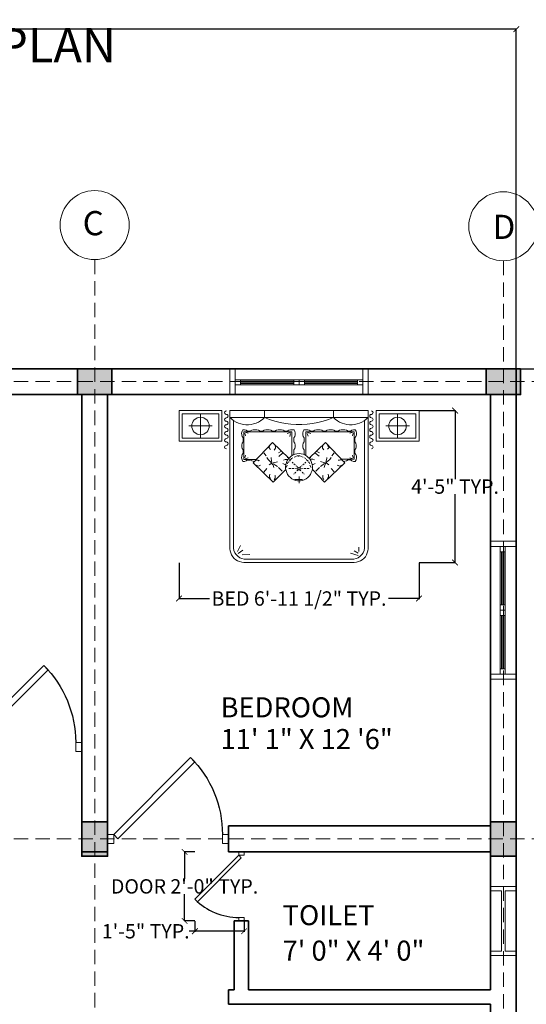
# Model space of a CAD drawing. Units: inches. Extents: x 782 to 2660, y -1008 to 166.
# Tile 10 of 12: x 1234 to 1410, y -176 to 166. Entities that reach past the tile are written whole.
import ezdxf

# ---------------------------------------------------------------- set-up
doc = ezdxf.new("R2010")
doc.units = ezdxf.units.IN
doc.header["$MEASUREMENT"] = 0
doc.linetypes.add('DASHED', pattern=[0.75, 0.5, -0.25])
for name, color, linetype, lineweight in [('A-ANNO-DIMS', 4, 'Continuous', 18), ('A-ANNO-TEXT', 4, 'Continuous', 18), ('A-AREA-IDEN', 4, 'Continuous', 18), ('A-COLS', 7, 'Continuous', 35), ('A-Door', 150, 'Continuous', 18), ('A-FURN', 8, 'Continuous', 13), ('A-Glaz', 4, 'Continuous', 18), ('A-GRID', 8, 'DASHED', 13), ('A-GRID-IDEN', 7, 'Continuous', 18), ('A-WALL', 7, 'Continuous', 35)]:
    doc.layers.add(name, color=color, linetype=linetype, lineweight=lineweight)
doc.layers.add('NET 01', color=8, linetype='Continuous')
doc.styles.get("Standard").update_dxf_attribs({"font": 'arial.ttf'})
doc.dimstyles.get("Standard").update_dxf_attribs({"dimtxt": 5, "dimasz": 2, "dimexe": 0.18, "dimexo": 0.0625, "dimgap": 0.09, "dimtad": 0, "dimtih": 1, "dimtoh": 1, "dimdec": 0, "dimzin": 0, "dimdsep": 46, "dimlunit": 3, "dimtxsty": 'Standard', "dimblk": 'ARCHTICK', "dimcen": 0.09, "dimadec": 0, "dimazin": 0, "dimtfac": 1, "dimtdec": 0, "dimtofl": 0, "dimtmove": 0, "dimatfit": 3, "dimfxl": 1, "dimtolj": 1, "dimtzin": 0, "dimarcsym": 0})

# ---------------------------------------------------------------- blocks, each defined once
blk = doc.blocks.new('A$C592222DF')
at = {"layer": 'A-Door'}
for points in [[(-0.0354, -0.0354), (-0.6718, 0.601), (-0.6364, 0.6364), (0, 0)], [(-0.95, 0), (-0.95, -0.075), (-0.9, -0.075), (-0.9, 0)], [(0, 0), (0, -0.075), (0.05, -0.075), (0.05, 0)]]:
    blk.add_lwpolyline(points, close=True, dxfattribs=at)
at = {"layer": 'NET 01'}
blk.add_arc((0, 0), 0.9, 135, 180, dxfattribs=at)
blk = doc.blocks.new('d-bed-4')
at = {"color": 0, "linetype": 'ByBlock'}
for p, q in [((0.56, 0), (0, 0)), ((0, 0), (0, -0.4)), ((0.56, -0.4), (0.56, 0)), ((0.664, -1.8), (0.664, 0)), ((0.664, 0), (2.464, 0)), ((0.664, 0), (2.464, 0)), ((0.664, -1.8), (0.664, 0)), ((1.114, 0), (1.114, -0.09)), ((2.014, 0), (2.014, -0.09)), ((2.464, 0), (2.464, -1.8)), ((2.464, 0), (2.464, -1.8)), ((2.568, -0.4), (2.568, 0)), ((2.568, 0), (3.128, 0)), ((3.128, 0), (3.128, -0.4)), ((0.52, -0.04), (0.04, -0.04)), ((0.04, -0.04), (0.04, -0.36)), ((0.28, -0.046), (0.28, -0.354)), ((0.52, -0.36), (0.52, -0.04)), ((2.464, -0.09), (0.664, -0.09)), ((0.664, -0.09), (0.689, -0.112)), ((0.689, -0.112), (0.716, -0.131)), ((0.709, -1.795), (0.709, -0.128)), ((1.064, -0.131), (1.091, -0.112)), ((1.091, -0.112), (1.114, -0.09)), ((1.114, -0.09), (1.181, -0.115)), ((1.181, -0.115), (1.249, -0.137)), ((1.879, -0.137), (1.947, -0.115)), ((1.947, -0.115), (2.014, -0.09)), ((2.014, -0.09), (2.037, -0.112)), ((2.037, -0.112), (2.064, -0.131)), ((2.412, -0.131), (2.439, -0.112)), ((2.419, -0.128), (2.419, -1.795)), ((2.439, -0.112), (2.464, -0.09)), ((2.608, -0.36), (2.608, -0.04)), ((2.608, -0.04), (3.088, -0.04)), ((2.848, -0.046), (2.848, -0.354)), ((3.088, -0.04), (3.088, -0.36)), ((0.126, -0.2), (0.434, -0.2)), ((0.716, -0.131), (0.745, -0.148)), ((0.745, -0.148), (0.776, -0.162)), ((0.776, -0.162), (0.806, -0.173)), ((0.806, -0.173), (0.84, -0.18)), ((0.821, -0.268), (0.831, -0.248)), ((0.831, -0.248), (0.853, -0.248)), ((0.84, -0.18), (0.873, -0.184)), ((0.853, -0.248), (0.875, -0.256)), ((0.873, -0.184), (0.907, -0.184)), ((0.875, -0.256), (0.894, -0.266)), ((0.907, -0.184), (0.939, -0.18)), ((0.925, -0.266), (0.947, -0.256)), ((0.939, -0.18), (0.972, -0.173)), ((0.947, -0.256), (0.968, -0.25)), ((0.968, -0.25), (0.99, -0.248)), ((0.972, -0.173), (1.004, -0.162)), ((0.99, -0.248), (1.013, -0.25)), ((1.004, -0.162), (1.035, -0.148)), ((1.013, -0.25), (1.035, -0.256)), ((1.035, -0.148), (1.064, -0.131)), ((1.035, -0.256), (1.056, -0.266)), ((1.087, -0.266), (1.109, -0.256)), ((1.109, -0.256), (1.13, -0.25)), ((1.13, -0.25), (1.152, -0.248)), ((1.152, -0.248), (1.175, -0.25)), ((1.175, -0.25), (1.197, -0.256)), ((1.197, -0.256), (1.217, -0.266)), ((1.249, -0.137), (1.317, -0.155)), ((1.249, -0.266), (1.269, -0.256)), ((1.269, -0.256), (1.29, -0.25)), ((1.29, -0.25), (1.314, -0.248)), ((1.314, -0.248), (1.337, -0.25)), ((1.317, -0.155), (1.388, -0.169)), ((1.337, -0.25), (1.359, -0.256)), ((1.359, -0.256), (1.379, -0.266)), ((1.388, -0.169), (1.458, -0.178)), ((1.411, -0.266), (1.431, -0.256)), ((1.431, -0.256), (1.451, -0.248)), ((1.451, -0.248), (1.474, -0.248)), ((1.458, -0.178), (1.528, -0.182)), ((1.474, -0.248), (1.501, -0.248)), ((1.501, -0.248), (1.51, -0.268)), ((1.528, -0.182), (1.6, -0.182)), ((1.6, -0.182), (1.67, -0.178)), ((1.627, -0.248), (1.618, -0.268)), ((1.654, -0.248), (1.627, -0.248)), ((1.677, -0.248), (1.654, -0.248)), ((1.67, -0.178), (1.74, -0.169)), ((1.697, -0.256), (1.677, -0.248)), ((1.717, -0.266), (1.697, -0.256)), ((1.74, -0.169), (1.811, -0.155)), ((1.769, -0.256), (1.749, -0.266)), ((1.791, -0.25), (1.769, -0.256)), ((1.814, -0.248), (1.791, -0.25)), ((1.811, -0.155), (1.879, -0.137)), ((1.838, -0.25), (1.814, -0.248)), ((1.859, -0.256), (1.838, -0.25)), ((1.879, -0.266), (1.859, -0.256)), ((1.931, -0.256), (1.911, -0.266)), ((1.953, -0.25), (1.931, -0.256)), ((1.976, -0.248), (1.953, -0.25)), ((1.998, -0.25), (1.976, -0.248)), ((2.019, -0.256), (1.998, -0.25)), ((2.041, -0.266), (2.019, -0.256)), ((2.064, -0.131), (2.093, -0.148)), ((2.093, -0.256), (2.072, -0.266)), ((2.093, -0.148), (2.124, -0.162)), ((2.115, -0.25), (2.093, -0.256)), ((2.138, -0.248), (2.115, -0.25)), ((2.124, -0.162), (2.156, -0.173)), ((2.16, -0.25), (2.138, -0.248)), ((2.156, -0.173), (2.189, -0.18)), ((2.181, -0.256), (2.16, -0.25)), ((2.203, -0.266), (2.181, -0.256)), ((2.189, -0.18), (2.221, -0.184)), ((2.221, -0.184), (2.255, -0.184)), ((2.253, -0.256), (2.234, -0.266)), ((2.275, -0.248), (2.253, -0.256)), ((2.255, -0.184), (2.288, -0.18)), ((2.297, -0.248), (2.275, -0.248)), ((2.288, -0.18), (2.322, -0.173)), ((2.307, -0.268), (2.297, -0.248)), ((2.322, -0.173), (2.352, -0.162)), ((2.352, -0.162), (2.383, -0.148)), ((2.383, -0.148), (2.412, -0.131)), ((3.002, -0.2), (2.694, -0.2)), ((0.04, -0.36), (0.52, -0.36)), ((0.815, -0.292), (0.821, -0.268)), ((0.817, -0.315), (0.815, -0.292)), ((0.824, -0.337), (0.817, -0.315)), ((0.835, -0.356), (0.824, -0.337)), ((0.835, -0.405), (0.835, -0.356)), ((0.844, -0.635), (0.844, -0.275)), ((0.844, -0.275), (1.472, -0.275)), ((0.857, -0.293), (0.866, -0.329)), ((0.862, -0.281), (0.902, -0.293)), ((0.894, -0.266), (0.925, -0.266)), ((1.056, -0.266), (1.087, -0.266)), ((1.217, -0.266), (1.249, -0.266)), ((1.379, -0.266), (1.411, -0.266)), ((1.451, -0.284), (1.409, -0.299)), ((1.454, -0.299), (1.445, -0.335)), ((1.472, -0.275), (1.472, -0.581)), ((1.508, -0.337), (1.496, -0.356)), ((1.496, -0.356), (1.496, -0.405)), ((1.515, -0.315), (1.508, -0.337)), ((1.51, -0.268), (1.515, -0.292)), ((1.515, -0.292), (1.515, -0.315)), ((1.618, -0.268), (1.613, -0.292)), ((1.613, -0.292), (1.613, -0.315)), ((1.613, -0.315), (1.62, -0.337)), ((1.62, -0.337), (1.632, -0.356)), ((1.632, -0.356), (1.632, -0.405)), ((2.282, -0.274), (1.654, -0.274)), ((1.654, -0.274), (1.654, -0.58)), ((1.672, -0.297), (1.681, -0.333)), ((1.676, -0.283), (1.717, -0.297)), ((1.749, -0.266), (1.717, -0.266)), ((1.911, -0.266), (1.879, -0.266)), ((2.072, -0.266), (2.041, -0.266)), ((2.234, -0.266), (2.203, -0.266)), ((2.264, -0.279), (2.225, -0.292)), ((2.27, -0.292), (2.261, -0.328)), ((2.282, -0.634), (2.282, -0.274)), ((2.293, -0.356), (2.304, -0.337)), ((2.293, -0.405), (2.293, -0.356)), ((2.304, -0.337), (2.311, -0.315)), ((2.313, -0.292), (2.307, -0.268)), ((2.311, -0.315), (2.313, -0.292)), ((3.088, -0.36), (2.608, -0.36)), ((0, -0.4), (0.56, -0.4)), ((0.819, -0.448), (0.824, -0.425)), ((0.819, -0.47), (0.819, -0.448)), ((0.824, -0.493), (0.819, -0.47)), ((0.824, -0.425), (0.835, -0.405)), ((0.835, -0.513), (0.824, -0.493)), ((0.835, -0.553), (0.835, -0.513)), ((0.965, -0.68), (1.217, -0.416)), ((1.19, -0.452), (1.172, -0.482)), ((1.172, -0.482), (1.193, -0.506)), ((1.217, -0.416), (1.433, -0.621)), ((1.256, -0.491), (1.238, -0.515)), ((1.253, -0.446), (1.256, -0.491)), ((1.496, -0.405), (1.508, -0.425)), ((1.508, -0.493), (1.496, -0.513)), ((1.496, -0.513), (1.496, -0.567)), ((1.508, -0.425), (1.514, -0.448)), ((1.514, -0.47), (1.508, -0.493)), ((1.514, -0.448), (1.514, -0.47)), ((1.62, -0.425), (1.614, -0.448)), ((1.614, -0.448), (1.614, -0.47)), ((1.614, -0.47), (1.62, -0.493)), ((1.632, -0.405), (1.62, -0.425)), ((1.62, -0.493), (1.632, -0.513)), ((1.632, -0.513), (1.632, -0.567)), ((1.91, -0.414), (1.694, -0.619)), ((1.874, -0.445), (1.87, -0.49)), ((1.87, -0.49), (1.888, -0.513)), ((2.162, -0.679), (1.91, -0.414)), ((1.955, -0.481), (1.933, -0.504)), ((1.937, -0.45), (1.955, -0.481)), ((2.304, -0.425), (2.293, -0.405)), ((2.293, -0.513), (2.304, -0.493)), ((2.293, -0.553), (2.293, -0.513)), ((2.309, -0.448), (2.304, -0.425)), ((2.304, -0.493), (2.309, -0.47)), ((2.309, -0.47), (2.309, -0.448)), ((3.128, -0.4), (2.568, -0.4)), ((0.815, -0.617), (0.817, -0.594)), ((0.821, -0.641), (0.815, -0.617)), ((0.817, -0.594), (0.824, -0.572)), ((0.831, -0.661), (0.821, -0.641)), ((0.824, -0.572), (0.835, -0.553)), ((1.01, -0.635), (0.844, -0.635)), ((0.857, -0.617), (0.866, -0.581)), ((0.862, -0.63), (0.902, -0.617)), ((1.105, -0.551), (1.136, -0.59)), ((1.163, -0.639), (1.145, -0.612)), ((1.202, -0.675), (1.163, -0.639)), ((1.199, -0.626), (1.199, -0.612)), ((1.211, -0.675), (1.199, -0.626)), ((1.328, -0.533), (1.298, -0.551)), ((1.355, -0.551), (1.301, -0.596)), ((1.382, -0.635), (1.361, -0.644)), ((1.415, -0.635), (1.382, -0.635)), ((1.409, -0.612), (1.433, -0.621)), ((1.411, -0.652), (1.425, -0.63)), ((1.415, -0.635), (1.418, -0.639)), ((1.425, -0.63), (1.443, -0.61)), ((1.465, -0.626), (1.438, -0.659)), ((1.438, -0.635), (1.442, -0.641)), ((1.443, -0.61), (1.463, -0.592)), ((1.463, -0.592), (1.487, -0.578)), ((1.465, -0.626), (1.483, -0.617)), ((1.487, -0.578), (1.512, -0.567)), ((1.528, -0.596), (1.501, -0.608)), ((1.512, -0.567), (1.537, -0.562)), ((1.537, -0.562), (1.564, -0.558)), ((1.537, -0.59), (1.562, -0.59)), ((1.58, -0.59), (1.555, -0.59)), ((1.559, -0.587), (1.559, -0.599)), ((1.559, -0.587), (1.559, -0.599)), ((1.564, -0.558), (1.591, -0.562)), ((1.589, -0.596), (1.616, -0.608)), ((1.591, -0.562), (1.616, -0.567)), ((1.616, -0.567), (1.641, -0.578)), ((1.652, -0.626), (1.634, -0.617)), ((1.641, -0.578), (1.665, -0.592)), ((1.659, -0.635), (1.681, -0.657)), ((1.665, -0.592), (1.685, -0.61)), ((1.685, -0.61), (1.703, -0.63)), ((1.717, -0.61), (1.694, -0.619)), ((1.703, -0.63), (1.717, -0.652)), ((1.712, -0.634), (1.708, -0.637)), ((1.712, -0.634), (1.744, -0.634)), ((1.744, -0.634), (1.766, -0.643)), ((1.771, -0.549), (1.825, -0.594)), ((1.798, -0.531), (1.829, -0.549)), ((1.915, -0.673), (1.928, -0.625)), ((1.924, -0.673), (1.964, -0.637)), ((1.928, -0.625), (1.928, -0.61)), ((1.964, -0.637), (1.982, -0.61)), ((2.021, -0.549), (1.991, -0.589)), ((2.117, -0.634), (2.282, -0.634)), ((2.264, -0.628), (2.225, -0.616)), ((2.27, -0.616), (2.261, -0.58)), ((2.304, -0.572), (2.293, -0.553)), ((2.297, -0.661), (2.307, -0.641)), ((2.311, -0.594), (2.304, -0.572)), ((2.307, -0.641), (2.313, -0.617)), ((2.313, -0.617), (2.311, -0.594)), ((0.853, -0.661), (0.831, -0.661)), ((0.875, -0.653), (0.853, -0.661)), ((0.894, -0.643), (0.875, -0.653)), ((0.907, -0.644), (0.893, -0.644)), ((0.925, -0.643), (0.894, -0.643)), ((0.916, -0.644), (0.907, -0.644)), ((0.925, -0.644), (0.916, -0.644)), ((0.947, -0.653), (0.925, -0.643)), ((0.968, -0.659), (0.947, -0.653)), ((1.229, -0.932), (0.965, -0.68)), ((0.983, -0.661), (0.968, -0.659)), ((1.006, -0.644), (1.024, -0.644)), ((1.006, -0.711), (1.037, -0.725)), ((1.024, -0.644), (1.042, -0.653)), ((1.042, -0.653), (1.028, -0.644)), ((1.028, -0.644), (1.051, -0.648)), ((1.037, -0.725), (1.055, -0.716)), ((1.055, -0.716), (1.064, -0.711)), ((1.105, -0.801), (1.145, -0.756)), ((1.175, -0.707), (1.208, -0.684)), ((1.22, -0.707), (1.211, -0.675)), ((1.226, -0.68), (1.283, -0.666)), ((1.226, -0.711), (1.235, -0.743)), ((1.229, -0.693), (1.283, -0.729)), ((1.343, -0.788), (1.298, -0.743)), ((1.379, -0.702), (1.352, -0.689)), ((1.379, -0.702), (1.391, -0.702)), ((1.389, -0.729), (1.393, -0.702)), ((1.389, -0.756), (1.389, -0.729)), ((1.395, -0.781), (1.389, -0.756)), ((1.393, -0.702), (1.4, -0.677)), ((1.397, -0.743), (1.411, -0.711)), ((1.4, -0.677), (1.411, -0.652)), ((1.42, -0.677), (1.415, -0.695)), ((1.42, -0.677), (1.429, -0.668)), ((1.46, -0.756), (1.429, -0.756)), ((1.487, -0.686), (1.474, -0.671)), ((1.496, -0.756), (1.474, -0.756)), ((1.514, -0.707), (1.496, -0.695)), ((1.514, -0.756), (1.51, -0.756)), ((1.532, -0.72), (1.523, -0.72)), ((1.55, -0.765), (1.523, -0.756)), ((1.559, -0.747), (1.537, -0.729)), ((1.55, -0.756), (1.55, -0.747)), ((1.55, -0.747), (1.559, -0.747)), ((1.55, -0.765), (1.55, -0.756)), ((1.559, -0.77), (1.55, -0.765)), ((1.559, -0.747), (1.562, -0.745)), ((1.568, -0.747), (1.562, -0.745)), ((1.568, -0.747), (1.589, -0.729)), ((1.577, -0.747), (1.568, -0.747)), ((1.568, -0.77), (1.577, -0.765)), ((1.577, -0.756), (1.577, -0.747)), ((1.577, -0.765), (1.577, -0.756)), ((1.577, -0.765), (1.604, -0.756)), ((1.595, -0.72), (1.604, -0.72)), ((1.613, -0.707), (1.631, -0.695)), ((1.613, -0.756), (1.616, -0.756)), ((1.631, -0.756), (1.652, -0.756)), ((1.64, -0.686), (1.652, -0.671)), ((1.667, -0.756), (1.697, -0.756)), ((1.697, -0.677), (1.688, -0.668)), ((1.697, -0.677), (1.703, -0.695)), ((1.721, -0.743), (1.706, -0.711)), ((1.717, -0.652), (1.728, -0.677)), ((1.728, -0.677), (1.735, -0.702)), ((1.739, -0.756), (1.733, -0.781)), ((1.748, -0.7), (1.735, -0.7)), ((1.735, -0.702), (1.739, -0.729)), ((1.739, -0.729), (1.739, -0.756)), ((1.897, -0.931), (1.739, -0.769)), ((1.748, -0.7), (1.775, -0.688)), ((1.784, -0.787), (1.829, -0.742)), ((1.901, -0.679), (1.843, -0.664)), ((1.897, -0.691), (1.843, -0.727)), ((1.901, -0.709), (1.892, -0.742)), ((1.897, -0.931), (2.162, -0.679)), ((1.906, -0.706), (1.915, -0.673)), ((1.951, -0.706), (1.919, -0.682)), ((2.021, -0.799), (1.982, -0.754)), ((2.072, -0.715), (2.063, -0.709)), ((2.09, -0.724), (2.072, -0.715)), ((2.099, -0.643), (2.075, -0.646)), ((2.102, -0.643), (2.084, -0.652)), ((2.084, -0.652), (2.099, -0.643)), ((2.12, -0.709), (2.09, -0.724)), ((2.12, -0.643), (2.102, -0.643)), ((2.145, -0.661), (2.16, -0.659)), ((2.16, -0.659), (2.181, -0.653)), ((2.181, -0.653), (2.203, -0.643)), ((2.201, -0.643), (2.21, -0.643)), ((2.203, -0.643), (2.234, -0.643)), ((2.21, -0.643), (2.219, -0.643)), ((2.219, -0.643), (2.234, -0.643)), ((2.234, -0.643), (2.253, -0.653)), ((2.253, -0.653), (2.275, -0.661)), ((2.275, -0.661), (2.297, -0.661)), ((1.181, -0.851), (1.184, -0.828)), ((1.181, -0.869), (1.181, -0.851)), ((1.193, -0.891), (1.181, -0.869)), ((1.229, -0.932), (1.388, -0.77)), ((1.238, -0.9), (1.253, -0.882)), ((1.253, -0.846), (1.247, -0.846)), ((1.253, -0.882), (1.253, -0.846)), ((1.404, -0.808), (1.395, -0.781)), ((1.415, -0.832), (1.404, -0.808)), ((1.431, -0.853), (1.415, -0.832)), ((1.451, -0.873), (1.431, -0.853)), ((1.47, -0.889), (1.451, -0.873)), ((1.496, -0.902), (1.47, -0.889)), ((1.501, -0.819), (1.496, -0.828)), ((1.609, -0.896), (1.503, -0.896)), ((1.523, -0.801), (1.51, -0.815)), ((1.532, -0.792), (1.532, -0.792)), ((1.559, -0.77), (1.537, -0.783)), ((1.559, -0.77), (1.562, -0.77)), ((1.568, -0.77), (1.562, -0.77)), ((1.564, -0.945), (1.564, -0.86)), ((1.568, -0.77), (1.589, -0.783)), ((1.595, -0.792), (1.595, -0.792)), ((1.604, -0.801), (1.616, -0.815)), ((1.625, -0.819), (1.631, -0.828)), ((1.658, -0.889), (1.632, -0.902)), ((1.677, -0.873), (1.658, -0.889)), ((1.697, -0.853), (1.677, -0.873)), ((1.713, -0.832), (1.697, -0.853)), ((1.724, -0.808), (1.713, -0.832)), ((1.733, -0.781), (1.724, -0.808)), ((1.874, -0.88), (1.874, -0.844)), ((1.874, -0.844), (1.879, -0.844)), ((1.888, -0.898), (1.874, -0.88)), ((1.933, -0.889), (1.946, -0.868)), ((1.946, -0.85), (1.942, -0.826)), ((1.946, -0.868), (1.946, -0.85)), ((1.521, -0.911), (1.496, -0.902)), ((1.546, -0.916), (1.521, -0.911)), ((1.564, -0.916), (1.546, -0.916)), ((1.582, -0.916), (1.564, -0.916)), ((1.607, -0.911), (1.582, -0.916)), ((1.632, -0.902), (1.607, -0.911)), ((0.716, -1.825), (0.709, -1.795)), ((0.763, -1.836), (0.803, -1.76)), ((2.342, -1.836), (2.342, -1.778)), ((2.419, -1.795), (2.412, -1.825)), ((0.668, -1.827), (0.664, -1.8)), ((0.668, -1.827), (0.664, -1.8)), ((0.675, -1.854), (0.668, -1.827)), ((0.675, -1.854), (0.668, -1.827)), ((0.686, -1.881), (0.675, -1.854)), ((0.686, -1.881), (0.675, -1.854)), ((0.7, -1.904), (0.686, -1.881)), ((0.7, -1.904), (0.686, -1.881)), ((0.718, -1.926), (0.7, -1.904)), ((0.718, -1.926), (0.7, -1.904)), ((0.727, -1.852), (0.716, -1.825)), ((0.745, -1.877), (0.727, -1.852)), ((0.767, -1.899), (0.745, -1.877)), ((0.792, -1.917), (0.767, -1.899)), ((0.772, -1.863), (0.83, -1.818)), ((0.819, -1.928), (0.792, -1.917)), ((0.821, -1.881), (0.925, -1.876)), ((2.333, -1.89), (2.234, -1.858)), ((2.333, -1.858), (2.282, -1.827)), ((2.336, -1.917), (2.309, -1.928)), ((2.361, -1.899), (2.336, -1.917)), ((2.383, -1.877), (2.361, -1.899)), ((2.401, -1.852), (2.383, -1.877)), ((2.412, -1.825), (2.401, -1.852)), ((2.428, -1.904), (2.41, -1.926)), ((2.428, -1.904), (2.41, -1.926)), ((2.442, -1.881), (2.428, -1.904)), ((2.442, -1.881), (2.428, -1.904)), ((2.453, -1.854), (2.442, -1.881)), ((2.453, -1.854), (2.442, -1.881)), ((2.46, -1.827), (2.453, -1.854)), ((2.46, -1.827), (2.453, -1.854)), ((2.464, -1.8), (2.46, -1.827)), ((2.464, -1.8), (2.46, -1.827)), ((0.74, -1.944), (0.718, -1.926)), ((0.74, -1.944), (0.718, -1.926)), ((0.763, -1.958), (0.74, -1.944)), ((0.763, -1.958), (0.74, -1.944)), ((0.79, -1.969), (0.763, -1.958)), ((0.79, -1.969), (0.763, -1.958)), ((0.817, -1.976), (0.79, -1.969)), ((0.817, -1.976), (0.79, -1.969)), ((0.844, -1.98), (0.817, -1.976)), ((0.844, -1.98), (0.817, -1.976)), ((0.849, -1.935), (0.819, -1.928)), ((2.284, -1.98), (0.844, -1.98)), ((2.284, -1.98), (0.844, -1.98)), ((2.279, -1.935), (0.849, -1.935)), ((2.309, -1.928), (2.279, -1.935)), ((2.311, -1.976), (2.284, -1.98)), ((2.311, -1.976), (2.284, -1.98)), ((2.338, -1.969), (2.311, -1.976)), ((2.338, -1.969), (2.311, -1.976)), ((2.365, -1.958), (2.338, -1.969)), ((2.365, -1.958), (2.338, -1.969)), ((2.388, -1.944), (2.365, -1.958)), ((2.388, -1.944), (2.365, -1.958)), ((2.41, -1.926), (2.388, -1.944)), ((2.41, -1.926), (2.388, -1.944))]:
    blk.add_line(p, q, dxfattribs=at)
for centre in [(0.28, -0.2), (2.848, -0.2)]:
    blk.add_ellipse(centre, major_axis=(-0.0806, 0.0806), ratio=1, dxfattribs=at)
for centre, major_axis, start_param, end_param in [((0.617, -0.026), (-0.0159, 0.0159), 5.497787, 8.63938), ((0.617, -0.116), (-0.0159, 0.0159), 5.497787, 8.63938), ((0.617, -0.071), (-0.0159, 0.0159), 2.356194, 5.497787), ((2.507, -0.071), (0.0159, 0.0159), 0.785398, 3.926991), ((2.507, -0.026), (0.0159, 0.0159), 3.926991, 7.068583), ((2.507, -0.116), (0.0159, 0.0159), 3.926991, 7.068583), ((0.617, -0.206), (-0.0159, 0.0159), 5.497787, 8.63938), ((0.617, -0.161), (-0.0159, 0.0159), 2.356194, 5.497787), ((0.617, -0.161), (-0.0159, 0.0159), 2.356194, 5.497787), ((0.617, -0.251), (-0.0159, 0.0159), 2.356194, 5.497787), ((2.507, -0.161), (0.0159, 0.0159), 0.785398, 3.926991), ((2.507, -0.161), (0.0159, 0.0159), 0.785398, 3.926991), ((2.507, -0.251), (0.0159, 0.0159), 0.785398, 3.926991), ((2.507, -0.206), (0.0159, 0.0159), 3.926991, 7.068583), ((0.617, -0.296), (-0.0159, 0.0159), 5.497787, 8.63938), ((0.617, -0.386), (-0.0159, 0.0159), 5.497787, 8.63938), ((0.617, -0.341), (-0.0159, 0.0159), 2.356194, 5.497787), ((2.507, -0.341), (0.0159, 0.0159), 0.785398, 3.926991), ((2.507, -0.296), (0.0159, 0.0159), 3.926991, 7.068583), ((2.507, -0.386), (0.0159, 0.0159), 3.926991, 7.068583), ((0.617, -0.476), (-0.0159, 0.0159), 5.497787, 8.63938), ((0.617, -0.431), (-0.0159, 0.0159), 2.356194, 5.497787), ((2.507, -0.431), (0.0159, 0.0159), 0.785398, 3.926991), ((2.507, -0.476), (0.0159, 0.0159), 3.926991, 7.068583)]:
    blk.add_ellipse(centre, major_axis=major_axis, ratio=1, start_param=start_param, end_param=end_param, dxfattribs=at)
blk = doc.blocks.new('WIN-48-FRAME-A')
for p, q in [((0, 48), (0, 0)), ((0, 48), (9, 48)), ((9, 48), (0, 48)), ((9, 48), (9, 0)), ((9, 46.15), (0, 46.15)), ((9, 46.15), (0, 46.15)), ((9, 46.15), (0, 46.15)), ((3.35, 1.85), (3.35, 46.15)), ((5.19, 1.85), (5.19, 46.15)), ((5.19, 44.31), (3.35, 44.31)), ((3.9, 44.31), (3.9, 25.85)), ((4.27, 44.31), (4.27, 25.85)), ((4.64, 44.31), (4.64, 25.85)), ((3.35, 25.85), (5.19, 25.85)), ((3.35, 24), (5.19, 24)), ((3.35, 22.15), (5.19, 22.15)), ((3.9, 3.69), (3.9, 22.15)), ((4.27, 3.69), (4.27, 22.15)), ((4.64, 3.69), (4.64, 22.15)), ((5.19, 3.69), (3.35, 3.69)), ((9, 1.85), (0, 1.85)), ((9, 1.85), (0, 1.85)), ((0, 0), (9, 0)), ((0, 0), (9, 0))]:
    blk.add_line(p, q)
blk = doc.blocks.new('WIN-24')
for p, q in [((0, 0), (0, 24)), ((0, 24), (9, 24)), ((9, 24), (9, 0)), ((0, 22.49), (3.9, 22.49)), ((3.9, 1.51), (3.9, 22.49)), ((5.1, 22.49), (9, 22.49)), ((5.1, 1.51), (5.1, 22.49)), ((3.9, 1.51), (0, 1.51)), ((9, 0), (0, 0)), ((9, 1.51), (5.1, 1.51))]:
    blk.add_line(p, q)
blk = doc.blocks.new('COL-9X12')
h = blk.add_hatch(color=256)
h.dxf.hatch_style = 1
h.paths.add_polyline_path([(9, 12), (0, 12), (0, 0), (9, 0)])
blk.add_lwpolyline([(0, 12), (9, 12), (9, 0), (0, 0)], close=True)
blk = doc.blocks.new('_ArchTick')
at = {"color": 0, "linetype": 'ByBlock', "const_width": 0.15}
blk.add_lwpolyline([(-0.5, -0.5), (0.5, 0.5)], dxfattribs=at)
blk = doc.blocks.new('*D29')
at = {"layer": 'A-ANNO-DIMS', "color": 0, "lineweight": -2, "transparency": 16777216}
for p, q in [((1294.95, -122.99), (1291.23, -122.99)), ((1291.41, -122.99), (1291.41, -132.32)), ((1291.41, -146.99), (1291.41, -137.67)), ((1294.95, -146.99), (1291.23, -146.99))]:
    blk.add_line(p, q, dxfattribs=at)
at = {"layer": 'Defpoints', "color": 0, "transparency": 16777216}
for p in [(1291.41, -122.99), (1295.01, -122.99), (1295.01, -146.99)]:
    blk.add_point(p, dxfattribs=at)
at = {"layer": 'A-ANNO-DIMS', "color": 0, "lineweight": -2, "transparency": 16777216, "xscale": 2, "yscale": 2, "zscale": 2}
for p, rotation in [((1291.41, -122.99), 90), ((1291.41, -146.99), 270)]:
    blk.add_blockref('_ArchTick', p, dxfattribs=dict(at, rotation=rotation))
at = {"layer": 'A-ANNO-DIMS', "color": 0, "transparency": 16777216, "insert": (1291.41, -134.99), "char_height": 5, "attachment_point": 5}
blk.add_mtext('\\A1;DOOR 2\'-0" TYP.', dxfattribs=at)
blk = doc.blocks.new('*D30')
at = {"layer": 'A-ANNO-DIMS', "color": 0, "lineweight": -2, "transparency": 16777216}
for p, q in [((1295.01, -147.06), (1295.01, -150.77)), ((1312.08, -147.06), (1312.08, -150.77)), ((1295.01, -150.59), (1293.01, -150.59)), ((1312.08, -150.59), (1295.01, -150.59))]:
    blk.add_line(p, q, dxfattribs=at)
at = {"layer": 'Defpoints', "color": 0, "transparency": 16777216}
for p in [(1295.01, -146.99), (1312.08, -146.99), (1295.01, -150.59)]:
    blk.add_point(p, dxfattribs=at)
at = {"layer": 'A-ANNO-DIMS', "color": 0, "lineweight": -2, "transparency": 16777216, "xscale": 2, "yscale": 2, "zscale": 2, "rotation": 180}
blk.add_blockref('_ArchTick', (1295.01, -150.59), dxfattribs=at)
at = {"layer": 'A-ANNO-DIMS', "color": 0, "lineweight": -2, "transparency": 16777216, "xscale": 2, "yscale": 2, "zscale": 2}
blk.add_blockref('_ArchTick', (1312.08, -150.59), dxfattribs=at)
at = {"layer": 'A-ANNO-DIMS', "color": 0, "transparency": 16777216, "insert": (1277.92, -150.59), "char_height": 5, "attachment_point": 5}
blk.add_mtext('\\A1;1\'-5" TYP.', dxfattribs=at)
blk = doc.blocks.new('*D41')
at = {"layer": 'A-ANNO-DIMS', "color": 0, "lineweight": -2, "transparency": 16777216}
for p, q in [((1289.48, -22.44), (1289.48, -35.07)), ((1372.89, -22.44), (1372.89, -35.07)), ((1289.48, -34.89), (1300.05, -34.89)), ((1372.89, -34.89), (1362.32, -34.89))]:
    blk.add_line(p, q, dxfattribs=at)
at = {"layer": 'Defpoints', "color": 0, "transparency": 16777216}
for p in [(1289.48, -22.37), (1372.89, -22.37), (1372.89, -34.89)]:
    blk.add_point(p, dxfattribs=at)
at = {"layer": 'A-ANNO-DIMS', "color": 0, "lineweight": -2, "transparency": 16777216, "xscale": 2, "yscale": 2, "zscale": 2, "rotation": 180}
blk.add_blockref('_ArchTick', (1289.48, -34.89), dxfattribs=at)
at = {"layer": 'A-ANNO-DIMS', "color": 0, "lineweight": -2, "transparency": 16777216, "xscale": 2, "yscale": 2, "zscale": 2}
blk.add_blockref('_ArchTick', (1372.89, -34.89), dxfattribs=at)
at = {"layer": 'A-ANNO-DIMS', "color": 0, "transparency": 16777216, "insert": (1331.18, -34.89), "char_height": 5, "attachment_point": 5}
blk.add_mtext('\\A1;BED 6\'-11 1/2" TYP.', dxfattribs=at)
blk = doc.blocks.new('*D42')
at = {"layer": 'A-ANNO-DIMS', "color": 0, "lineweight": -2, "transparency": 16777216}
for p, q in [((1372.95, 30.43), (1385.58, 30.43)), ((1385.4, 30.43), (1385.4, 6.66)), ((1385.4, -22.37), (1385.4, 1.39)), ((1372.95, -22.37), (1385.58, -22.37))]:
    blk.add_line(p, q, dxfattribs=at)
at = {"layer": 'Defpoints', "color": 0, "transparency": 16777216}
for p in [(1372.89, 30.43), (1385.4, 30.43), (1372.89, -22.37)]:
    blk.add_point(p, dxfattribs=at)
at = {"layer": 'A-ANNO-DIMS', "color": 0, "lineweight": -2, "transparency": 16777216, "xscale": 2, "yscale": 2, "zscale": 2}
for p, rotation in [((1385.4, 30.43), 90), ((1385.4, -22.37), 270)]:
    blk.add_blockref('_ArchTick', p, dxfattribs=dict(at, rotation=rotation))
at = {"layer": 'A-ANNO-DIMS', "color": 0, "transparency": 16777216, "insert": (1385.4, 4.03), "char_height": 5, "attachment_point": 5}
blk.add_mtext('\\A1;4\'-5" TYP.', dxfattribs=at)
blk = doc.blocks.new('*D51')
at = {"layer": 'A-ANNO-DIMS', "color": 0, "lineweight": -2, "transparency": 16777216}
for p, q in [((1406.75, 45.01), (1579.89, 45.01)), ((1579.71, 45.01), (1579.71, -327.35)), ((1579.71, -704.99), (1579.71, -332.64)), ((1406.75, -704.99), (1579.89, -704.99))]:
    blk.add_line(p, q, dxfattribs=at)
at = {"layer": 'Defpoints', "color": 0, "transparency": 16777216}
for p in [(1406.68, 45.01), (1579.71, 45.01), (1406.68, -704.99)]:
    blk.add_point(p, dxfattribs=at)
at = {"layer": 'A-ANNO-DIMS', "color": 0, "lineweight": -2, "transparency": 16777216, "xscale": 2, "yscale": 2, "zscale": 2}
for p, rotation in [((1579.71, 45.01), 90), ((1579.71, -704.99), 270)]:
    blk.add_blockref('_ArchTick', p, dxfattribs=dict(at, rotation=rotation))
at = {"layer": 'A-ANNO-DIMS', "color": 0, "transparency": 16777216, "insert": (1579.71, -329.99), "char_height": 5, "attachment_point": 5}
blk.add_mtext('\\A1;62\'-6"', dxfattribs=at)
blk = doc.blocks.new('*D52')
at = {"layer": 'A-ANNO-DIMS', "color": 0, "lineweight": -2, "transparency": 16777216}
for p, q in [((982.68, 45.07), (982.68, 163.27)), ((982.68, 163.09), (1186.01, 163.09)), ((1406.68, 163.09), (1203.36, 163.09)), ((1406.68, 45.07), (1406.68, 163.27))]:
    blk.add_line(p, q, dxfattribs=at)
at = {"layer": 'Defpoints', "color": 0, "transparency": 16777216}
for p in [(1406.68, 163.09), (982.68, 45.01), (1406.68, 45.01)]:
    blk.add_point(p, dxfattribs=at)
at = {"layer": 'A-ANNO-DIMS', "color": 0, "lineweight": -2, "transparency": 16777216, "xscale": 2, "yscale": 2, "zscale": 2, "rotation": 180}
blk.add_blockref('_ArchTick', (982.68, 163.09), dxfattribs=at)
at = {"layer": 'A-ANNO-DIMS', "color": 0, "lineweight": -2, "transparency": 16777216, "xscale": 2, "yscale": 2, "zscale": 2}
blk.add_blockref('_ArchTick', (1406.68, 163.09), dxfattribs=at)
at = {"layer": 'A-ANNO-DIMS', "color": 0, "transparency": 16777216, "insert": (1194.68, 163.09), "char_height": 5, "attachment_point": 5}
blk.add_mtext('\\A1;35\'-4"', dxfattribs=at)

msp = doc.modelspace()

# ---------------------------------------------------------------- linework, layer by layer
at = {"layer": 'A-GRID', "ltscale": 10}
for p, q in [((1260.18, 82.94), (1260.18, -927.11)), ((1402.18, 82.53), (1402.18, -937.14)), ((1499.56, 40.51), (955.26, 40.51)), ((1499.56, -118.49), (876.32, -118.49))]:
    msp.add_line(p, q, dxfattribs=at)
at = {"layer": 'A-GRID-IDEN'}
for centre in [(1260.18, 94.94), (1402.18, 94.53)]:
    msp.add_circle(centre, 12, dxfattribs=at)
at = {"layer": 'A-WALL'}
for p, q in [((982.68, 45.01), (1406.68, 45.01)), ((1406.68, 45.01), (1406.68, -476.99)), ((1107.68, 36.01), (1255.68, 36.01)), ((1255.68, 36.01), (1255.68, -83.99)), ((1264.68, 36.01), (1264.68, -113.99)), ((1264.68, 36.01), (1397.68, 36.01)), ((1397.68, 36.01), (1397.68, -113.99)), ((1255.68, -83.99), (1255.68, -88.99)), ((1255.68, -88.99), (1255.68, -122.99)), ((1264.68, -113.99), (1264.68, -122.99)), ((1306.68, -113.99), (1397.68, -113.99)), ((1306.68, -113.99), (1306.68, -122.99)), ((1255.68, -122.99), (1264.68, -122.99)), ((1306.68, -122.99), (1308.68, -122.99)), ((1308.68, -122.99), (1313.68, -122.99)), ((1313.68, -122.99), (1397.68, -122.99)), ((1397.68, -122.99), (1397.68, -170.99)), ((1308.68, -146.99), (1308.68, -170.99)), ((1308.68, -146.99), (1313.68, -146.99)), ((1313.68, -146.99), (1313.68, -170.99)), ((1306.68, -175.99), (1306.68, -170.99)), ((1306.68, -170.99), (1308.68, -170.99)), ((1313.68, -170.99), (1397.68, -170.99)), ((1306.68, -175.99), (1397.68, -175.99)), ((1397.68, -175.99), (1397.68, -284.99))]:
    msp.add_line(p, q, dxfattribs=at)

# ---------------------------------------------------------------- block references
at = {"layer": 'A-COLS'}
for p, rotation in [((1254.18, 45.01), 270.0000000000027), ((1396.18, 45.01), 270.0000000000018), ((1406.68, -112.49), 180)]:
    msp.add_blockref('COL-9X12', p, dxfattribs=dict(at, rotation=rotation))
msp.add_blockref('COL-9X12', (1255.68, -124.49), dxfattribs=at)
at = {"layer": 'A-Door', "xscale": -42, "yscale": 42, "zscale": 42}
for p in [(1215.78, -84.92), (1266.78, -116.92)]:
    msp.add_blockref('A$C592222DF', p, dxfattribs=at)
at = {"layer": 'A-Door', "xscale": 24, "yscale": 24, "zscale": 24, "rotation": 90}
msp.add_blockref('A$C592222DF', (1310.28, -124.19), dxfattribs=at)
at = {"layer": 'A-FURN', "xscale": 26.66666775212405, "yscale": 26.66666775212405, "zscale": 26.66666775212405}
msp.add_blockref('d-bed-4', (1289.48, 30.43), dxfattribs=at)
at = {"layer": 'A-Glaz', "rotation": 90.00000000000036}
msp.add_blockref('WIN-48-FRAME-A', (1355.18, 36.01), dxfattribs=at)
at = {"layer": 'A-Glaz'}
for name, p in [('WIN-48-FRAME-A', (1397.68, -62.99)), ('WIN-24', (1397.68, -158.99))]:
    msp.add_blockref(name, p, dxfattribs=at)

# ---------------------------------------------------------------- texts
at = {"layer": 'A-ANNO-TEXT'}
msp.add_text('GROUND FLOOR PLAN', height=11.9654, dxfattribs=at).set_placement((1098.34, 151.5))
at = {"layer": 'A-AREA-IDEN'}
for s, height, p in [('BEDROOM', 6.958, (1303.93, -76.21)), ('11\' 1" X 12 \'6"', 6.9576, (1303.93, -87.23)), ('TOILET', 6.958, (1325.48, -148.48)), ('7\' 0" X 4\' 0"', 6.9576, (1325.48, -160.81))]:
    msp.add_text(s, height=height, dxfattribs=at).set_placement(p)
at = {"layer": 'A-GRID-IDEN'}
for s, p in [('C', (1256.02, 91.42)), ('D', (1398.45, 90.13))]:
    msp.add_text(s, height=8.41, dxfattribs=at).set_placement(p)

# ---------------------------------------------------------------- dimensions: what is measured, and where the dimension line sits
at = {"layer": 'A-ANNO-DIMS'}
dim = msp.add_linear_dim(base=(1406.68, 163.09), p1=(982.68, 45.01), p2=(1406.68, 45.01), dimstyle='Standard', override={"dimdec": 1, "dimlfac": 1, "dimrnd": 0, "dimzin": 1, "dimdsep": 46, "dimlunit": 4, "dimfrac": 2}, dxfattribs=at)
dim.commit()
dim.dimension.update_dxf_attribs({"geometry": '*D52', "text_midpoint": (1194.68, 163.09)})
dim = msp.add_linear_dim(base=(1579.71, 45.01), p1=(1406.68, -704.99), p2=(1406.68, 45.01), angle=90, dimstyle='Standard', override={"dimdec": 1, "dimlfac": 1, "dimrnd": 0, "dimzin": 1, "dimdsep": 46, "dimlunit": 4, "dimfrac": 2}, dxfattribs=at)
dim.commit()
dim.dimension.update_dxf_attribs({"geometry": '*D51', "text_midpoint": (1579.71, -329.99)})
for base, p1, p2, angle, text, picture, middle in [((1385.4, 30.43), (1372.89, -22.37), (1372.89, 30.43), 90, '<> TYP.', '*D42', (1385.4, 4.03)), ((1291.41, -122.99), (1295.01, -146.99), (1295.01, -122.99), 90, 'DOOR <> TYP.', '*D29', (1291.41, -134.99)), ((1295.01, -150.59), (1312.08, -146.99), (1295.01, -146.99), 180, '<> TYP.', '*D30', (1277.92, -150.59))]:
    dim = msp.add_linear_dim(base=base, p1=p1, p2=p2, angle=angle, text=text, dimstyle='Standard', override={"dimdec": 1, "dimlfac": 1, "dimrnd": 0, "dimzin": 1, "dimdsep": 46, "dimlunit": 4, "dimfrac": 2}, dxfattribs=at)
    dim.commit()
    dim.dimension.update_dxf_attribs({"geometry": picture, "text_midpoint": middle})
dim = msp.add_linear_dim(base=(1372.89, -34.89), p1=(1289.48, -22.37), p2=(1372.89, -22.37), text='BED <> TYP.', dimstyle='Standard', override={"dimdec": 1, "dimlfac": 1, "dimrnd": 0, "dimzin": 1, "dimdsep": 46, "dimlunit": 4, "dimfrac": 2}, dxfattribs=at)
dim.commit()
dim.dimension.update_dxf_attribs({"geometry": '*D41', "text_midpoint": (1331.18, -34.89)})

doc.saveas('drawing.dxf')
